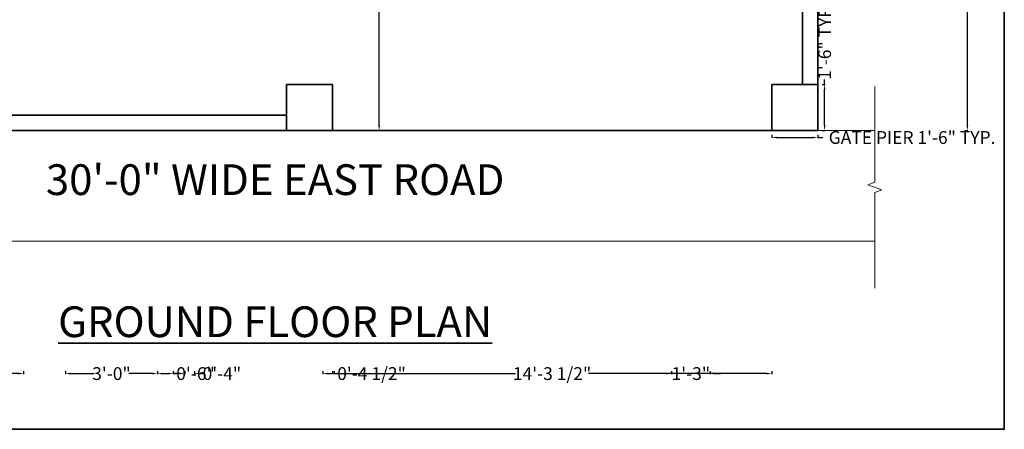
# Model space of a CAD drawing. Units: inches. Extents: x -231 to 349, y -511 to 252.
# Tile 2 of 6: x -36 to 349, y -511 to -351. Entities that reach past the tile are written whole.
import ezdxf

# ---------------------------------------------------------------- set-up
doc = ezdxf.new("R2010")
doc.units = ezdxf.units.IN
doc.header["$MEASUREMENT"] = 0
for name, color, linetype, lineweight in [('A-ANNO-DIMS', 7, 'Continuous', 18), ('A-ANNO-TEXT', 7, 'Continuous', 18), ('A-ANNO-TTLB', 7, 'Continuous', 35), ('C-PROP', 7, 'Continuous', 35), ('C-ROAD', 8, 'Continuous', 18)]:
    doc.layers.add(name, color=color, linetype=linetype, lineweight=lineweight)
doc.styles.get("Standard").update_dxf_attribs({"font": 'arial.ttf'})
doc.dimstyles.get("Standard").update_dxf_attribs({"dimtxt": 5, "dimasz": 2, "dimexe": 0.18, "dimexo": 0.0625, "dimgap": 0.09, "dimtad": 0, "dimzin": 0, "dimdsep": 46, "dimlunit": 4, "dimtxsty": 'Standard', "dimcen": 0.09, "dimadec": 0, "dimazin": 0, "dimtfac": 1, "dimtofl": 0, "dimtmove": 0, "dimatfit": 3, "dimfxl": 1, "dimfxlon": 1, "dimtolj": 1, "dimtzin": 0, "dimarcsym": 0})

# ---------------------------------------------------------------- blocks, each defined once
blk = doc.blocks.new('*D26')
at = {"layer": 'A-ANNO-DIMS', "color": 0, "lineweight": -2, "transparency": 16777216}
for p, q in [((105.45, -186.12), (104.27, -186.12)), ((104.45, -188.12), (104.45, -280.1)), ((104.45, -392.62), (104.45, -300.64)), ((105.45, -394.62), (104.27, -394.62))]:
    blk.add_line(p, q, dxfattribs=at)
at = {"layer": 'A-ANNO-DIMS', "color": 0, "transparency": 16777216}
for points in [[(104.12, -188.12), (104.79, -188.12), (104.45, -186.12)], [(104.12, -392.62), (104.79, -392.62), (104.45, -394.62)]]:
    blk.add_solid(points, dxfattribs=at)
at = {"layer": 'Defpoints', "color": 0, "transparency": 16777216}
for p in [(104.45, -186.12), (115.6, -186.12), (115.6, -394.62)]:
    blk.add_point(p, dxfattribs=at)
at = {"layer": 'A-ANNO-DIMS', "color": 0, "transparency": 16777216, "insert": (104.45, -290.37), "char_height": 5, "attachment_point": 5, "rotation": 90}
blk.add_mtext('\\A1;17\'-4{\\H1x;\\S1/2;}"', dxfattribs=at)
blk = doc.blocks.new('GATE-PIER-18IN')
for p, q in [((275.92, -376.62), (257.92, -376.62)), ((257.92, -376.62), (257.92, -394.62)), ((275.92, -394.62), (275.92, -376.62))]:
    blk.add_line(p, q)
blk = doc.blocks.new('*D32')
at = {"layer": 'A-ANNO-DIMS', "color": 0, "lineweight": -2, "transparency": 16777216}
for p, q in [((257.92, -396.32), (257.92, -397.5)), ((275.92, -396.32), (275.92, -397.5)), ((259.92, -397.32), (273.92, -397.32)), ((275.92, -397.32), (277.92, -397.32))]:
    blk.add_line(p, q, dxfattribs=at)
at = {"layer": 'A-ANNO-DIMS', "color": 0, "transparency": 16777216}
for points in [[(259.92, -396.99), (259.92, -397.65), (257.92, -397.32)], [(273.92, -396.99), (273.92, -397.65), (275.92, -397.32)]]:
    blk.add_solid(points, dxfattribs=at)
at = {"layer": 'Defpoints', "color": 0, "transparency": 16777216}
for p in [(257.92, -394.62), (275.92, -394.62), (275.92, -397.32)]:
    blk.add_point(p, dxfattribs=at)
at = {"layer": 'A-ANNO-DIMS', "color": 0, "transparency": 16777216, "insert": (312.81, -397.32), "char_height": 5, "attachment_point": 5}
blk.add_mtext('\\A1;GATE PIER 1\'-6" TYP.', dxfattribs=at)
blk = doc.blocks.new('*D33')
at = {"layer": 'A-ANNO-DIMS', "color": 0, "lineweight": -2, "transparency": 16777216}
for p, q in [((277.62, -376.62), (278.8, -376.62)), ((278.62, -376.62), (278.62, -374.62)), ((278.62, -392.62), (278.62, -378.62)), ((277.62, -394.62), (278.8, -394.62))]:
    blk.add_line(p, q, dxfattribs=at)
at = {"layer": 'A-ANNO-DIMS', "color": 0, "transparency": 16777216}
for points in [[(278.29, -378.62), (278.95, -378.62), (278.62, -376.62)], [(278.29, -392.62), (278.95, -392.62), (278.62, -394.62)]]:
    blk.add_solid(points, dxfattribs=at)
at = {"layer": 'Defpoints', "color": 0, "transparency": 16777216}
for p in [(275.92, -376.62), (278.62, -376.62), (275.92, -394.62)]:
    blk.add_point(p, dxfattribs=at)
at = {"layer": 'A-ANNO-DIMS', "color": 0, "transparency": 16777216, "insert": (278.62, -359.53), "char_height": 5, "attachment_point": 5, "rotation": 90}
blk.add_mtext('\\A1;1\'-6" TYP.', dxfattribs=at)
blk = doc.blocks.new('*D45')
at = {"layer": 'A-ANNO-DIMS', "color": 0, "lineweight": -2, "transparency": 16777216}
for p, q in [((333.44, 181.38), (334.62, 181.38)), ((334.44, 179.38), (334.44, -97.84)), ((334.44, -392.62), (334.44, -115.4)), ((333.44, -394.62), (334.62, -394.62))]:
    blk.add_line(p, q, dxfattribs=at)
at = {"layer": 'A-ANNO-DIMS', "color": 0, "transparency": 16777216}
for points in [[(334.11, 179.38), (334.78, 179.38), (334.44, 181.38)], [(334.11, -392.62), (334.78, -392.62), (334.44, -394.62)]]:
    blk.add_solid(points, dxfattribs=at)
at = {"layer": 'Defpoints', "color": 0, "transparency": 16777216}
for p in [(275.92, 181.38), (275.92, -394.62), (334.44, -394.62)]:
    blk.add_point(p, dxfattribs=at)
at = {"layer": 'A-ANNO-DIMS', "color": 0, "transparency": 16777216, "insert": (334.44, -106.62), "char_height": 5, "attachment_point": 5, "rotation": 90}
blk.add_mtext('\\A1;48\'-0"', dxfattribs=at)
blk = doc.blocks.new('*D48')
at = {"layer": 'A-ANNO-DIMS', "color": 0, "lineweight": -2, "transparency": 16777216}
for p, q in [((86.18, -488.55), (86.18, -489.73)), ((257.92, -488.55), (257.92, -489.73)), ((88.18, -489.55), (157.78, -489.55)), ((255.92, -489.55), (186.32, -489.55))]:
    blk.add_line(p, q, dxfattribs=at)
at = {"layer": 'A-ANNO-DIMS', "color": 0, "transparency": 16777216}
for points in [[(88.18, -489.21), (88.18, -489.88), (86.18, -489.55)], [(255.92, -489.21), (255.92, -489.88), (257.92, -489.55)]]:
    blk.add_solid(points, dxfattribs=at)
at = {"layer": 'Defpoints', "color": 0, "transparency": 16777216}
for p in [(86.18, -394.62), (257.92, -394.62), (257.92, -489.55)]:
    blk.add_point(p, dxfattribs=at)
at = {"layer": 'A-ANNO-DIMS', "color": 0, "transparency": 16777216, "insert": (172.05, -489.55), "char_height": 5, "attachment_point": 5}
blk.add_mtext('\\A1;14\'-3 1/2"', dxfattribs=at)
blk = doc.blocks.new('*D51')
at = {"layer": 'A-ANNO-DIMS', "color": 0, "lineweight": -2, "transparency": 16777216}
for p, q in [((28.42, -488.55), (28.42, -489.73)), ((32.24, -488.55), (32.24, -489.73)), ((26.42, -489.55), (24.42, -489.55)), ((34.24, -489.55), (36.24, -489.55))]:
    blk.add_line(p, q, dxfattribs=at)
at = {"layer": 'A-ANNO-DIMS', "color": 0, "transparency": 16777216}
for points in [[(26.42, -489.21), (26.42, -489.88), (28.42, -489.55)], [(34.24, -489.21), (34.24, -489.88), (32.24, -489.55)]]:
    blk.add_solid(points, dxfattribs=at)
at = {"layer": 'Defpoints', "color": 0, "transparency": 16777216}
for p in [(28.42, 133.38), (32.24, 133.38), (32.24, -489.55)]:
    blk.add_point(p, dxfattribs=at)
at = {"layer": 'A-ANNO-DIMS', "color": 0, "transparency": 16777216, "insert": (42.97, -489.55), "char_height": 5, "attachment_point": 5}
blk.add_mtext('\\A1;0\'-4"', dxfattribs=at)
blk = doc.blocks.new('*D56')
at = {"layer": 'A-ANNO-DIMS', "color": 0, "lineweight": -2, "transparency": 16777216}
for p, q in [((-96.08, -488.55), (-96.08, -489.73)), ((-34.58, -488.55), (-34.58, -489.73)), ((-94.08, -489.55), (-77.89, -489.55)), ((-36.58, -489.55), (-52.77, -489.55))]:
    blk.add_line(p, q, dxfattribs=at)
at = {"layer": 'A-ANNO-DIMS', "color": 0, "transparency": 16777216}
for points in [[(-94.08, -489.21), (-94.08, -489.88), (-96.08, -489.55)], [(-36.58, -489.21), (-36.58, -489.88), (-34.58, -489.55)]]:
    blk.add_solid(points, dxfattribs=at)
at = {"layer": 'Defpoints', "color": 0, "transparency": 16777216}
for p in [(-96.08, -334.62), (-34.58, -334.62), (-34.58, -489.55)]:
    blk.add_point(p, dxfattribs=at)
at = {"layer": 'A-ANNO-DIMS', "color": 0, "transparency": 16777216, "insert": (-65.33, -489.55), "char_height": 5, "attachment_point": 5}
blk.add_mtext('\\A1;5\'-1 1/2"', dxfattribs=at)
blk = doc.blocks.new('*D57')
at = {"layer": 'A-ANNO-DIMS', "color": 0, "lineweight": -2, "transparency": 16777216}
for p, q in [((218.71, -488.55), (218.71, -489.73)), ((233.92, -488.55), (233.92, -489.73)), ((216.71, -489.55), (214.71, -489.55)), ((235.92, -489.55), (237.92, -489.55))]:
    blk.add_line(p, q, dxfattribs=at)
at = {"layer": 'A-ANNO-DIMS', "color": 0, "transparency": 16777216}
for points in [[(216.71, -489.21), (216.71, -489.88), (218.71, -489.55)], [(235.92, -489.21), (235.92, -489.88), (233.92, -489.55)]]:
    blk.add_solid(points, dxfattribs=at)
at = {"layer": 'Defpoints', "color": 0, "transparency": 16777216}
for p in [(218.71, -186.12), (233.92, -186.12), (233.92, -489.55)]:
    blk.add_point(p, dxfattribs=at)
at = {"layer": 'A-ANNO-DIMS', "color": 0, "transparency": 16777216, "insert": (226.31, -489.55), "char_height": 5, "attachment_point": 5}
blk.add_mtext('\\A1;1\'-3"', dxfattribs=at)
blk = doc.blocks.new('*D58')
at = {"layer": 'A-ANNO-DIMS', "color": 0, "lineweight": -2, "transparency": 16777216}
for p, q in [((-18.2, -488.55), (-18.2, -489.73)), ((17.8, -488.55), (17.8, -489.73)), ((-16.2, -489.55), (-6.93, -489.55)), ((15.8, -489.55), (6.54, -489.55))]:
    blk.add_line(p, q, dxfattribs=at)
at = {"layer": 'A-ANNO-DIMS', "color": 0, "transparency": 16777216}
for points in [[(-16.2, -489.21), (-16.2, -489.88), (-18.2, -489.55)], [(15.8, -489.21), (15.8, -489.88), (17.8, -489.55)]]:
    blk.add_solid(points, dxfattribs=at)
at = {"layer": 'Defpoints', "color": 0, "transparency": 16777216}
for p in [(-18.2, -33.12), (17.8, -33.12), (17.8, -489.55)]:
    blk.add_point(p, dxfattribs=at)
at = {"layer": 'A-ANNO-DIMS', "color": 0, "transparency": 16777216, "insert": (-0.2, -489.55), "char_height": 5, "attachment_point": 5}
blk.add_mtext('\\A1;3\'-0"', dxfattribs=at)
blk = doc.blocks.new('*D59')
at = {"layer": 'A-ANNO-DIMS', "color": 0, "lineweight": -2, "transparency": 16777216}
for p, q in [((17.8, -488.55), (17.8, -489.73)), ((23.92, -488.55), (23.92, -489.73)), ((19.8, -489.55), (21.92, -489.55)), ((23.92, -489.55), (25.92, -489.55))]:
    blk.add_line(p, q, dxfattribs=at)
at = {"layer": 'A-ANNO-DIMS', "color": 0, "transparency": 16777216}
for points in [[(19.8, -489.21), (19.8, -489.88), (17.8, -489.55)], [(21.92, -489.21), (21.92, -489.88), (23.92, -489.55)]]:
    blk.add_solid(points, dxfattribs=at)
at = {"layer": 'Defpoints', "color": 0, "transparency": 16777216}
for p in [(17.8, -28.62), (23.92, -33.12), (23.92, -489.55)]:
    blk.add_point(p, dxfattribs=at)
at = {"layer": 'A-ANNO-DIMS', "color": 0, "transparency": 16777216, "insert": (32.66, -489.55), "char_height": 5, "attachment_point": 5}
blk.add_mtext('\\A1;0\'-6"', dxfattribs=at)
blk = doc.blocks.new('*D60')
at = {"layer": 'A-ANNO-DIMS', "color": 0, "lineweight": -2, "transparency": 16777216}
for p, q in [((82.42, -488.55), (82.42, -489.73)), ((86.92, -488.55), (86.92, -489.73)), ((84.42, -489.55), (84.92, -489.55)), ((86.92, -489.55), (88.92, -489.55))]:
    blk.add_line(p, q, dxfattribs=at)
at = {"layer": 'A-ANNO-DIMS', "color": 0, "transparency": 16777216}
for points in [[(84.42, -489.21), (84.42, -489.88), (82.42, -489.55)], [(84.92, -489.21), (84.92, -489.88), (86.92, -489.55)]]:
    blk.add_solid(points, dxfattribs=at)
at = {"layer": 'Defpoints', "color": 0, "transparency": 16777216}
for p in [(82.42, -33.12), (86.92, -33.12), (86.92, -489.55)]:
    blk.add_point(p, dxfattribs=at)
at = {"layer": 'A-ANNO-DIMS', "color": 0, "transparency": 16777216, "insert": (101.48, -489.55), "char_height": 5, "attachment_point": 5}
blk.add_mtext('\\A1;0\'-4 1/2"', dxfattribs=at)

msp = doc.modelspace()

# ---------------------------------------------------------------- linework, layer by layer
at = {"layer": 'A-ANNO-TTLB'}
msp.add_lwpolyline([(-231.158, 252.428), (348.864, 252.428), (348.864, -511.312), (-231.158, -511.312)], close=True, dxfattribs=at)
at = {"layer": 'C-PROP'}
for p, q in [((275.92, 181.38), (275.92, -394.62)), ((269.92, 175.38), (269.92, -376.62)), ((68.175, -388.62), (-150.08, -388.62)), ((275.92, -394.62), (-156.08, -394.62))]:
    msp.add_line(p, q, dxfattribs=at)
at = {"layer": 'C-ROAD'}
for p, q in [((275.92, -394.62), (298.295, -394.62)), ((298.295, -437.796), (-183.047, -437.796))]:
    msp.add_line(p, q, dxfattribs=at)
msp.add_lwpolyline([(298.295, -377.404), (298.295, -414.776), (295.547, -415.776), (301.042, -417.776), (298.295, -418.776), (298.295, -456.148)], dxfattribs=at)

# ---------------------------------------------------------------- block references
at = {"layer": 'C-PROP'}
for p in [(-189.744, 0), (0, 0)]:
    msp.add_blockref('GATE-PIER-18IN', p, dxfattribs=at)

# ---------------------------------------------------------------- texts
at = {"layer": 'A-ANNO-TEXT', "insert": (-38.131, -407.791), "char_height": 12, "attachment_point": 1}
msp.add_mtext_dynamic_manual_height_columns('\\pxqc;30\'-0" WIDE EAST ROAD', width=203.87214, gutter_width=1, heights=[0], dxfattribs=at)
at = {"layer": 'A-ANNO-TTLB', "insert": (-38.131, -463.3), "char_height": 12, "attachment_point": 1}
msp.add_mtext_dynamic_manual_height_columns('\\pxqc;{\\fArial|b1|i0|c0|p34;\\LGROUND FLOOR PLAN}', width=203.87214, gutter_width=1, heights=[0], dxfattribs=at)

# ---------------------------------------------------------------- dimensions: what is measured, and where the dimension line sits
at = {"layer": 'A-ANNO-DIMS'}
for base, p1, p2, override, picture, middle in [((334.442, -394.62), (275.92, 181.38), (275.92, -394.62), {"dimdec": 1, "dimlfac": 1, "dimrnd": 0, "dimzin": 1, "dimdsep": 46, "dimlunit": 4, "dimfrac": 2}, '*D45', (334.442, -106.62)), ((104.455, -186.12), (115.598, -394.62), (115.598, -186.12), {"dimclrd": 0, "dimclre": 0, "dimclrt": 0}, '*D26', (104.455, -290.37))]:
    dim = msp.add_linear_dim(base=base, p1=p1, p2=p2, angle=90, dimstyle='Standard', override=override, dxfattribs=at)
    dim.commit()
    dim.dimension.update_dxf_attribs({"geometry": picture, "text_midpoint": middle})
for base, p1, p2, picture, middle in [((32.236, -489.548), (28.42, 133.38), (32.236, 133.38), '*D51', (42.971, -489.548)), ((23.92, -489.548), (17.803, -28.62), (23.92, -33.12), '*D59', (32.655, -489.548)), ((17.803, -489.548), (-18.197, -33.12), (17.803, -33.12), '*D58', (-0.197, -489.548)), ((86.92, -489.548), (82.42, -33.12), (86.92, -33.12), '*D60', (101.481, -489.548)), ((233.92, -489.548), (218.708, -186.12), (233.92, -186.12), '*D57', (226.314, -489.548)), ((-34.58, -489.548), (-96.08, -334.62), (-34.58, -334.62), '*D56', (-65.33, -489.548)), ((257.92, -489.548), (86.175, -394.62), (257.92, -394.62), '*D48', (172.047, -489.548))]:
    dim = msp.add_linear_dim(base=base, p1=p1, p2=p2, dimstyle='Standard', override={"dimdec": 1, "dimlfac": 1, "dimrnd": 0, "dimzin": 1, "dimdsep": 46, "dimlunit": 4, "dimfrac": 2}, dxfattribs=at)
    dim.commit()
    dim.dimension.update_dxf_attribs({"geometry": picture, "text_midpoint": middle})
dim = msp.add_linear_dim(base=(278.62, -376.62), p1=(275.92, -394.62), p2=(275.92, -376.62), angle=90, text='<> TYP.', dimstyle='Standard', override={"dimdec": 1, "dimlfac": 1, "dimrnd": 0, "dimzin": 1, "dimdsep": 46, "dimlunit": 4, "dimfrac": 2}, dxfattribs=at)
dim.commit()
dim.dimension.update_dxf_attribs({"geometry": '*D33', "text_midpoint": (278.62, -359.527)})
dim = msp.add_linear_dim(base=(275.92, -397.32), p1=(257.92, -394.62), p2=(275.92, -394.62), text='GATE PIER <> TYP.', dimstyle='Standard', override={"dimdec": 1, "dimlfac": 1, "dimrnd": 0, "dimzin": 1, "dimdsep": 46, "dimlunit": 4, "dimfrac": 2}, dxfattribs=at)
dim.commit()
dim.dimension.update_dxf_attribs({"geometry": '*D32', "text_midpoint": (312.808, -397.32)})

doc.saveas('drawing.dxf')
